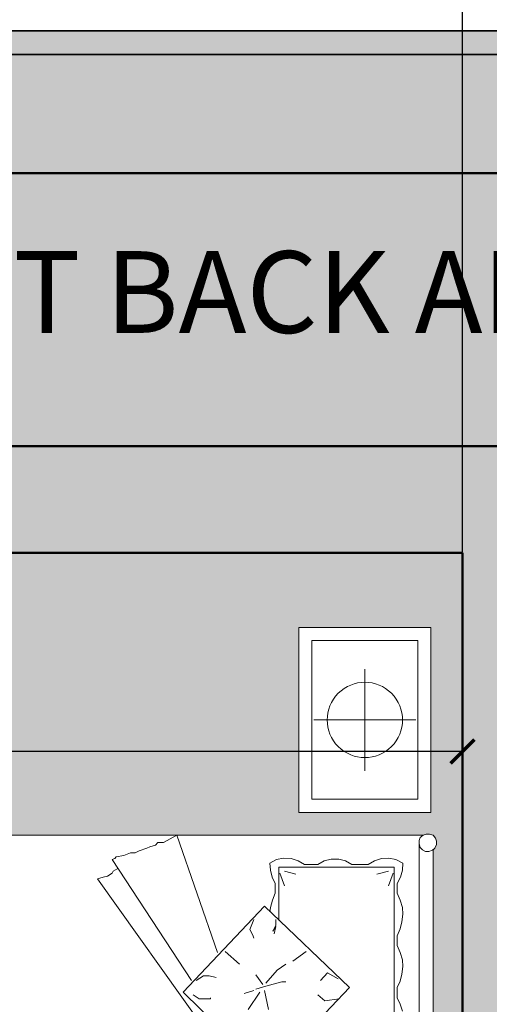
# Model space of a CAD drawing. Units: inches. Extents: x 528 to 2620, y -1066 to 798.
# Tile 16 of 41: x 737 to 776, y 672 to 755. Entities that reach past the tile are written whole.
import ezdxf

# ---------------------------------------------------------------- set-up
doc = ezdxf.new("R2010")
doc.units = ezdxf.units.IN
doc.header["$MEASUREMENT"] = 0
for name, color, linetype, lineweight in [('A-ANNO-DIMS', 2, 'Continuous', 18), ('A-AREA-IDEN', 7, 'Continuous', 18), ('A-FURN', 30, 'Continuous', 18), ('A-WALL', 7, 'Continuous', 50), ('A-WALL-PATT', 8, 'Continuous', 13), ('C-PROP', 5, 'Continuous', 35)]:
    doc.layers.add(name, color=color, linetype=linetype, lineweight=lineweight)
doc.styles.get("Standard").update_dxf_attribs({"font": 'arial.ttf'})
doc.dimstyles.get("Standard").update_dxf_attribs({"dimtxt": 6, "dimasz": 2, "dimexe": 0.18, "dimexo": 0.0625, "dimgap": 0.09, "dimtad": 0, "dimtih": 1, "dimtoh": 1, "dimdec": 1, "dimzin": 0, "dimdsep": 46, "dimlunit": 3, "dimtxsty": 'Standard', "dimblk": 'ARCHTICK', "dimcen": 0.09, "dimadec": 0, "dimazin": 0, "dimtfac": 1, "dimtdec": 1, "dimtofl": 0, "dimtmove": 0, "dimatfit": 3, "dimfxl": 1, "dimtolj": 1, "dimtzin": 0, "dimarcsym": 0})

# ---------------------------------------------------------------- blocks, each defined once
blk = doc.blocks.new('d-bed-3')
at = {"color": 0, "linetype": 'ByBlock'}
for p, q in [((0, 0), (0, -0.5)), ((0.7, 0), (0, 0)), ((0.7, -0.5), (0.7, 0)), ((0.7817, -0.0054), (0.7857, 0.0078)), ((0.7817, -0.0054), (0.7857, 0.0078)), ((0.7857, 0.0078), (0.7968, 0.0166)), ((0.7857, 0.0078), (0.7968, 0.0166)), ((0.7968, 0.0166), (0.8078, 0.0211)), ((0.7968, 0.0166), (0.8078, 0.0211)), ((0.8078, 0.0211), (0.8209, 0.0211)), ((0.8078, 0.0211), (0.8209, 0.0211)), ((0.8209, 0.0211), (0.8349, 0.0144)), ((0.8209, 0.0211), (0.8349, 0.0144)), ((0.8349, 0.0144), (0.8409, 0.0078)), ((0.8349, 0.0144), (0.8429, 0.0056)), ((0.8389, 0.0078), (2.7305, 0.0078)), ((0.8409, 0.0078), (2.7305, 0.0078)), ((0.8429, 0.0056), (0.848, -0.0077)), ((0.7817, -0.0187), (0.7817, -0.0054)), ((0.7817, -0.0187), (0.7817, -0.0054)), ((0.7857, -0.0297), (0.7817, -0.0187)), ((0.7857, -0.0297), (0.7817, -0.0187)), ((0.7857, -2.0939), (0.7857, -0.0297)), ((0.7948, -0.0408), (0.7857, -0.0297)), ((0.7857, -0.032), (0.7857, -2.0939)), ((0.8409, -0.032), (0.8319, -0.0408)), ((0.848, -0.0209), (0.8409, -0.032)), ((0.848, -0.0077), (0.848, -0.0209)), ((0.05, -0.05), (0.05, -0.45)), ((0.65, -0.05), (0.05, -0.05)), ((0.35, -0.0576), (0.35, -0.4424)), ((0.65, -0.45), (0.65, -0.05)), ((0.8058, -0.0452), (0.7948, -0.0408)), ((0.8188, -0.0452), (0.8058, -0.0452)), ((0.8319, -0.0408), (0.8188, -0.0452)), ((2.7525, -0.0452), (0.8188, -0.0452)), ((0.8781, -0.1325), (0.8911, -0.1059)), ((0.8911, -0.1059), (0.9182, -0.1082)), ((0.9182, -0.1082), (0.9443, -0.1148)), ((1.0317, -0.117), (1.0588, -0.1082)), ((1.0588, -0.1082), (1.0849, -0.1059)), ((1.0849, -0.1059), (1.113, -0.1104)), ((1.113, -0.1104), (1.1401, -0.117)), ((1.2295, -0.117), (1.2566, -0.1082)), ((1.2566, -0.1082), (1.2827, -0.1059)), ((1.2827, -0.1059), (1.3108, -0.1104)), ((1.3108, -0.1104), (1.3379, -0.117)), ((1.4253, -0.117), (1.4514, -0.1082)), ((0.8721, -0.159), (0.8781, -0.1325)), ((0.9072, -0.5753), (0.9072, -0.1391)), ((0.9072, -0.1391), (1.6763, -0.1391)), ((0.9293, -0.1435), (0.9775, -0.1612)), ((0.9443, -0.1148), (0.9684, -0.128)), ((0.9684, -0.128), (1.0056, -0.128)), ((1.0056, -0.128), (1.0317, -0.117)), ((1.1401, -0.117), (1.1662, -0.128)), ((1.1662, -0.128), (1.2034, -0.128)), ((1.2034, -0.128), (1.2295, -0.117)), ((1.3379, -0.117), (1.362, -0.128)), ((1.362, -0.128), (1.4012, -0.128)), ((1.4012, -0.128), (1.4253, -0.117)), ((0.8741, -0.1866), (0.8721, -0.159)), ((0.9223, -0.1612), (0.9333, -0.2042)), ((0.8831, -0.2131), (0.8741, -0.1866)), ((0.8962, -0.2374), (0.8831, -0.2131)), ((0.1576, -0.25), (0.5424, -0.25)), ((0.8962, -0.2992), (0.8962, -0.2374)), ((0.8761, -0.3489), (0.8831, -0.3235)), ((0.8831, -0.3235), (0.8962, -0.2992)), ((1.0538, -0.6294), (1.362, -0.3081)), ((1.362, -0.3081), (1.619, -0.5532)), ((0.8761, -0.3776), (0.8761, -0.3489)), ((1.3289, -0.3511), (1.3068, -0.3909)), ((1.4052, -0.3467), (1.4122, -0.4019)), ((0.8831, -0.4041), (0.8761, -0.3776)), ((0.8962, -0.4284), (0.8831, -0.4041)), ((1.3068, -0.3909), (1.3349, -0.4174)), ((1.4122, -0.4019), (1.3901, -0.4284)), ((0.8962, -0.4781), (0.8962, -0.4284)), ((0.05, -0.45), (0.65, -0.45)), ((0.8831, -0.5024), (0.8962, -0.4781)), ((1.2255, -0.4715), (1.2626, -0.5223)), ((0, -0.5), (0.7, -0.5)), ((0.8741, -0.5289), (0.8831, -0.5024)), ((0.9223, -0.5532), (0.9333, -0.5113)), ((0.8721, -0.5576), (0.8741, -0.5289)), ((0.8781, -0.5841), (0.8721, -0.5576)), ((0.9293, -0.5709), (0.9775, -0.5532)), ((1.2957, -0.5819), (1.2737, -0.5488)), ((1.3399, -0.5643), (1.3399, -0.5488)), ((0.8911, -0.6096), (0.8781, -0.5841)), ((1.109, -0.5753), (0.9072, -0.5753)), ((0.9684, -0.5886), (0.9443, -0.6007)), ((1.0056, -0.5886), (0.9684, -0.5886)), ((1.0317, -0.5996), (1.0056, -0.5886)), ((1.105, -0.5864), (1.1271, -0.5864)), ((1.1271, -0.5864), (1.1482, -0.5974)), ((1.1482, -0.5974), (1.1311, -0.5864)), ((1.1311, -0.5864), (1.1592, -0.593)), ((1.3459, -0.625), (1.2957, -0.5819)), ((1.357, -0.625), (1.3399, -0.5643)), ((0.9182, -0.6073), (0.8911, -0.6096)), ((0.9443, -0.6007), (0.9182, -0.6073)), ((1.0588, -0.6073), (1.0317, -0.5996)), ((1.3791, -0.9365), (1.0538, -0.6294)), ((1.0759, -0.6096), (1.0588, -0.6073)), ((1.368, -0.6626), (1.357, -0.625)), ((1.3731, -0.6294), (1.4453, -0.614)), ((1.105, -0.6692), (1.1421, -0.6846)), ((1.1642, -0.6736), (1.1753, -0.6692)), ((1.3138, -0.6626), (1.351, -0.6361)), ((1.3731, -0.6692), (1.3841, -0.7067)), ((1.3791, -0.6471), (1.4453, -0.6913)), ((1.1421, -0.6846), (1.1642, -0.6736)), ((1.2255, -0.7785), (1.2737, -0.7244)), ((1.3791, -0.9365), (1.5357, -0.7763)), ((0.7857, -0.9607), (1.2295, -0.8072)), ((0.9504, -1.2611), (1.5708, -0.8183)), ((1.3178, -0.8382), (1.3239, -0.8117)), ((1.3178, -0.8602), (1.3178, -0.8382)), ((1.4052, -0.8337), (1.4012, -0.8337)), ((1.4052, -0.8768), (1.4052, -0.8337)), ((1.3349, -0.8879), (1.3178, -0.8602)), ((1.3901, -0.8989), (1.4052, -0.8768)), ((0.8781, -1.2059), (1.3349, -0.9055)), ((0.8128, -1.0115), (0.7857, -0.9607)), ((0.8128, -1.0325), (0.8128, -1.0115)), ((0.8239, -1.0414), (0.8128, -1.0325)), ((0.8299, -1.0635), (0.8239, -1.0414)), ((0.8349, -1.0745), (0.8299, -1.0635)), ((0.845, -1.1032), (0.8349, -1.0745)), ((0.852, -1.1187), (0.845, -1.1032)), ((0.852, -1.1363), (0.852, -1.1187)), ((0.863, -1.1617), (0.852, -1.1363)), ((0.867, -1.1905), (0.863, -1.1617)), ((0.8741, -1.1949), (0.867, -1.1905)), ((0.9223, -1.2015), (0.9112, -1.1838)), ((0.8781, -1.2059), (0.8741, -1.1949)), ((0.9293, -1.2059), (0.9223, -1.2015)), ((0.9403, -1.2236), (0.9293, -1.2059)), ((0.9443, -1.2391), (0.9403, -1.2236)), ((0.9504, -1.2611), (0.9443, -1.2391))]:
    blk.add_line(p, q, dxfattribs=at)
blk.add_ellipse((0.35, -0.25), major_axis=(-0.1007, 0.1007), ratio=1, dxfattribs=at)
blk = doc.blocks.new('_ArchTick')
at = {"color": 0, "linetype": 'ByBlock', "const_width": 0.15}
blk.add_lwpolyline([(-0.5, -0.5), (0.5, 0.5)], dxfattribs=at)
blk = doc.blocks.new('*D11')
at = {"layer": 'A-ANNO-DIMS', "color": 0, "lineweight": -2, "transparency": 16777216}
for p, q in [((584.059, 753.985), (584.059, 794.007)), ((584.059, 793.827), (758.88, 793.827)), ((944.059, 793.827), (769.239, 793.827)), ((944.059, 753.985), (944.059, 794.007))]:
    blk.add_line(p, q, dxfattribs=at)
at = {"layer": 'Defpoints', "color": 0, "transparency": 16777216}
for p in [(944.059, 793.827), (584.059, 753.922), (944.059, 753.922)]:
    blk.add_point(p, dxfattribs=at)
at = {"layer": 'A-ANNO-DIMS', "color": 0, "lineweight": -2, "transparency": 16777216, "xscale": 2, "yscale": 2, "zscale": 2, "rotation": 180}
blk.add_blockref('_ArchTick', (584.059, 793.827), dxfattribs=at)
at = {"layer": 'A-ANNO-DIMS', "color": 0, "lineweight": -2, "transparency": 16777216, "xscale": 2, "yscale": 2, "zscale": 2}
blk.add_blockref('_ArchTick', (944.059, 793.827), dxfattribs=at)
at = {"layer": 'A-ANNO-DIMS', "color": 0, "transparency": 16777216, "insert": (764.059, 793.827), "char_height": 6, "attachment_point": 5}
blk.add_mtext("\\A1;30'", dxfattribs=at)
blk = doc.blocks.new('*D25')
at = {"layer": 'A-ANNO-DIMS', "color": 0, "lineweight": -2, "transparency": 16777216}
for p, q in [((629.059, 693.763), (629.059, 693.001)), ((629.059, 693.181), (687.951, 693.181)), ((774.059, 693.181), (715.168, 693.181)), ((774.059, 693.763), (774.059, 693.001))]:
    blk.add_line(p, q, dxfattribs=at)
at = {"layer": 'Defpoints', "color": 0, "transparency": 16777216}
for p in [(629.059, 693.826), (774.059, 693.826), (774.059, 693.181)]:
    blk.add_point(p, dxfattribs=at)
at = {"layer": 'A-ANNO-DIMS', "color": 0, "lineweight": -2, "transparency": 16777216, "xscale": 2, "yscale": 2, "zscale": 2, "rotation": 180}
blk.add_blockref('_ArchTick', (629.059, 693.181), dxfattribs=at)
at = {"layer": 'A-ANNO-DIMS', "color": 0, "lineweight": -2, "transparency": 16777216, "xscale": 2, "yscale": 2, "zscale": 2}
blk.add_blockref('_ArchTick', (774.059, 693.181), dxfattribs=at)
at = {"layer": 'A-ANNO-DIMS', "color": 0, "transparency": 16777216, "insert": (701.559, 693.181), "char_height": 6, "attachment_point": 5}
blk.add_mtext('\\A1;12\'-1.0"', dxfattribs=at)
blk = doc.blocks.new('*D56')
at = {"layer": 'A-ANNO-DIMS', "color": 0, "lineweight": -2, "transparency": 16777216}
for p, q in [((774.059, 709.985), (774.059, 788.102)), ((774.059, 787.922), (778.559, 787.922)), ((778.559, 709.985), (778.559, 788.102)), ((778.559, 787.922), (780.559, 787.922))]:
    blk.add_line(p, q, dxfattribs=at)
at = {"layer": 'Defpoints', "color": 0, "transparency": 16777216}
for p in [(778.559, 787.922), (774.059, 709.922), (778.559, 709.922)]:
    blk.add_point(p, dxfattribs=at)
at = {"layer": 'A-ANNO-DIMS', "color": 0, "lineweight": -2, "transparency": 16777216, "xscale": 2, "yscale": 2, "zscale": 2, "rotation": 180}
blk.add_blockref('_ArchTick', (774.059, 787.922), dxfattribs=at)
at = {"layer": 'A-ANNO-DIMS', "color": 0, "lineweight": -2, "transparency": 16777216, "xscale": 2, "yscale": 2, "zscale": 2}
blk.add_blockref('_ArchTick', (778.559, 787.922), dxfattribs=at)
at = {"layer": 'A-ANNO-DIMS', "color": 0, "transparency": 16777216, "insert": (795.615, 787.922), "char_height": 6, "attachment_point": 5}
blk.add_mtext('\\A1;0\'-4 1/2"', dxfattribs=at)

msp = doc.modelspace()

# ---------------------------------------------------------------- hatches: boundary and pattern name
at = {"layer": 'A-WALL-PATT', "transparency": 33554687}
h = msp.add_hatch(color=256, dxfattribs=at)
h.dxf.hatch_style = 1
h.paths.add_polyline_path([(944.059, 753.922), (584.059, 753.922), (584.059, 208.922), (608.059, 208.922), (608.059, 210.922), (586.059, 210.922), (586.059, 751.922), (942.059, 751.922), (942.059, 210.922), (728.059, 210.922), (728.059, 208.922), (944.059, 208.922)])
h = msp.add_hatch(color=256, dxfattribs=at)
h.dxf.hatch_style = 1
h.paths.add_polyline_path([(942.059, 751.922), (586.059, 751.922), (586.059, 210.922), (608.059, 210.922), (608.059, 220.922), (596.059, 220.922), (596.059, 741.922), (932.059, 741.922), (932.059, 220.922), (770.059, 220.922), (728.059, 220.922), (728.059, 210.922), (942.059, 210.922)])
at = {"layer": 'A-WALL-PATT', "transparency": 33554475}
h = msp.add_hatch(color=256, dxfattribs=at)
h.dxf.hatch_style = 1
h.paths.add_polyline_path([(620.059, 718.922), (908.059, 718.922), (908.059, 268.922), (770.059, 268.922), (770.059, 220.922), (932.059, 220.922), (932.059, 741.922), (596.059, 741.922), (596.059, 391.422), (620.059, 391.422)])
at = {"layer": 'A-WALL-PATT', "transparency": 33554687}
h = msp.add_hatch(color=256, dxfattribs=at)
h.dxf.hatch_style = 1
h.paths.add_polyline_path([(861.059, 273.922), (817.059, 273.922), (817.059, 272.922), (861.059, 272.922)])
h.paths.add_polyline_path([(817.059, 277.922), (815.059, 277.922), (815.059, 268.922), (817.059, 268.922)])
h.paths.add_polyline_path([(908.059, 397.922), (899.059, 397.922), (899.059, 395.922), (908.059, 395.922)])
h.paths.add_polyline_path([(908.059, 443.922), (899.059, 443.922), (899.059, 441.922), (908.059, 441.922)])
h.paths.add_polyline_path([(904.059, 441.922), (903.059, 441.922), (903.059, 397.922), (904.059, 397.922)])
h.paths.add_polyline_path([(625.059, 561.422), (624.059, 561.422), (624.059, 537.422), (625.059, 537.422)])
h.paths.add_polyline_path([(648.747, 334.444), (720.045, 334.444), (720.045, 344.998), (648.747, 344.998)], flags=9)
h.paths.add_polyline_path([(819.733, 323.153), (880.328, 323.153), (880.328, 333.708), (819.733, 333.708)], flags=9)
h.paths.add_polyline_path([(779.898, 680.607), (821.764, 680.607), (821.764, 691.169), (779.898, 691.169)], flags=9)
h.paths.add_polyline_path([(779.876, 692.362), (817.138, 692.362), (817.138, 703.058), (779.876, 703.058)], flags=9)
h.paths.add_polyline_path([(799.994, 453.884), (860.589, 453.884), (860.589, 464.439), (799.994, 464.439)], flags=9)
h.paths.add_polyline_path([(650.866, 539.397), (708.781, 539.397), (708.781, 549.952), (650.866, 549.952)], flags=9)
h.paths.add_polyline_path([(788.504, 612.01), (849.099, 612.01), (849.099, 622.565), (788.504, 622.565)], flags=9)
h.paths.add_polyline_path([(639.539, 648.31), (700.134, 648.31), (700.134, 658.865), (639.539, 658.865)], flags=9)
h.paths.add_polyline_path([(648.913, 346.09), (747.706, 346.09), (747.706, 356.778), (648.913, 356.778)], flags=9)
h.paths.add_polyline_path([(676.857, 450.66), (746.735, 450.66), (746.735, 461.355), (676.857, 461.355)], flags=9)
h.paths.add_polyline_path([(819.711, 334.947), (865.526, 334.947), (865.526, 345.636), (819.711, 345.636)], flags=9)
h.paths.add_polyline_path([(806.298, 467.745), (874.047, 467.745), (874.047, 478.441), (806.298, 478.441)], flags=9)
h.paths.add_polyline_path([(653.235, 552.284), (690.497, 552.284), (690.497, 562.979), (653.235, 562.979)], flags=9)
h.paths.add_polyline_path([(789.903, 623.407), (843.208, 623.407), (843.208, 634.103), (789.903, 634.103)], flags=9)
h.paths.add_polyline_path([(639.773, 662.103), (693.077, 662.103), (693.077, 672.798), (639.773, 672.798)], flags=9)
h.paths.add_polyline_path([(801.587, 242.914), (846.334, 242.914), (846.334, 253.603), (801.587, 253.603)], flags=9)
h.paths.add_polyline_path([(925.362, 593.982), (925.362, 674.057), (914.673, 674.057), (914.673, 593.982)], flags=9)
h.paths.add_polyline_path([(612.559, 593.982), (612.559, 674.057), (601.871, 674.057), (601.871, 593.982)], flags=9)
h.paths.add_polyline_path([(723.31, 726.564), (803.385, 726.564), (803.385, 737.252), (723.31, 737.252)], flags=9)
at = {"layer": 'A-WALL-PATT', "transparency": 33554521}
h = msp.add_hatch(color=256, dxfattribs=at)
h.dxf.hatch_style = 1
h.paths.add_polyline_path([(629.059, 709.922), (677.559, 709.922), (677.559, 718.922), (620.059, 718.922), (620.059, 667.922), (629.059, 667.922)])
h.paths.add_polyline_path([(790.559, 718.922), (725.559, 718.922), (725.559, 709.922), (774.059, 709.922), (774.059, 577.922), (768.481, 577.922), (768.559, 573.422), (774.059, 573.422), (774.059, 567.422), (778.559, 567.422), (778.559, 669.422), (831.059, 669.422), (831.059, 675.922), (826.559, 675.922), (826.559, 673.922), (778.559, 673.922), (778.559, 709.922), (790.559, 709.922)])
h.paths.add_polyline_path([(908.059, 718.922), (879.059, 718.922), (879.059, 709.922), (899.059, 709.922), (899.059, 641.672), (908.059, 641.672)])
h.paths.add_polyline_path([(629.059, 619.922), (620.059, 619.922), (620.059, 561.422), (629.059, 561.422), (629.059, 573.422), (724.059, 573.422), (724.059, 569.422), (728.559, 569.422), (728.559, 577.922), (629.059, 577.922)])
h.paths.add_polyline_path([(779.059, 391.422), (779.059, 400.422), (770.059, 400.422), (764.059, 400.422), (764.059, 397.422), (764.059, 391.422), (770.059, 391.422), (770.059, 268.922), (815.059, 268.922), (815.059, 277.922), (779.059, 277.922), (779.059, 359.767)])
h.paths.add_polyline_path([(908.059, 395.922), (899.059, 395.922), (851.059, 395.922), (851.059, 391.422), (899.059, 391.422), (899.059, 277.922), (863.059, 277.922), (863.059, 268.922), (908.059, 268.922)])
h.paths.add_polyline_path([(908.059, 593.672), (899.059, 593.672), (899.059, 525.422), (778.559, 525.422), (778.559, 527.172), (774.059, 527.172), (774.059, 520.922), (899.059, 520.922), (899.059, 443.922), (908.059, 443.922)])
h.paths.add_polyline_path([(629.059, 520.922), (728.559, 520.922), (728.559, 545.422), (724.059, 545.422), (724.059, 525.422), (629.059, 525.422), (629.059, 537.422), (620.059, 537.422), (620.059, 484.672), (629.059, 484.672)])
h.paths.add_polyline_path([(629.059, 436.672), (620.059, 436.672), (620.059, 391.422), (648.559, 391.422), (648.559, 400.422), (629.059, 400.422)])
h.paths.add_polyline_path([(716.059, 397.422), (716.059, 400.422), (696.559, 400.422), (696.559, 391.422), (716.059, 391.422)])
at = {"layer": 'A-WALL-PATT', "transparency": 33554590}
h = msp.add_hatch(color=256, dxfattribs=at)
h.dxf.hatch_style = 1
h.paths.add_polyline_path([(774.059, 709.922), (629.059, 709.922), (629.059, 577.922), (728.559, 577.922), (728.559, 579.422), (728.559, 619.422), (730.309, 619.422), (730.309, 619.384, -0.401453), (768.559, 579.422), (768.559, 577.922), (774.059, 577.922)])
h.paths.add_polyline_path([(723.896, 686.058), (723.968, 686.064), (723.828, 686.128)], flags=0)
h.paths.add_polyline_path([(722.785, 642.699), (722.893, 642.756), (722.893, 684.992), (722.647, 685.244), (722.647, 685.82), (723.079, 686.262), (723.533, 686.262), (723.968, 686.064), (724.739, 686.128), (770.696, 686.128), (770.78, 686.14), (771.126, 686.266), (771.694, 686.094), (771.94, 685.478), (771.67, 684.904), (771.582, 684.871), (771.582, 642.782), (771.878, 642.514), (771.878, 641.921), (771.511, 641.462), (770.855, 641.462), (770.401, 641.833), (770.401, 641.551), (724.739, 641.551), (723.991, 641.705), (723.443, 641.414), (722.879, 641.585), (722.597, 642.142)], flags=16)
h.paths.add_polyline_path([(723.994, 641.704), (723.994, 641.707), (723.991, 641.705)], flags=0)
h.paths.add_polyline_path([(722.893, 642.732), (722.893, 684.992), (722.647, 685.244), (722.647, 685.82), (723.079, 686.262), (723.287, 686.262), (722.991, 686.172), (722.794, 685.971), (722.647, 685.68), (722.647, 685.434), (722.745, 685.143), (722.942, 684.942), (723.238, 684.807), (723.484, 684.807), (723.779, 684.897), (723.976, 685.098), (724.174, 685.488), (724.124, 685.635), (724.124, 685.249), (723.631, 684.746), (723.631, 642.961), (724.124, 642.514), (724.124, 641.887), (723.656, 641.462), (723.079, 641.462), (722.647, 641.904), (722.647, 642.48)], flags=0)
h.paths.add_polyline_path([(722.647, 642.29), (722.647, 642.044), (722.794, 641.753), (723.079, 641.462), (723.287, 641.462), (722.879, 641.585), (722.597, 642.142)], flags=0)
h.paths.add_polyline_path([(770.745, 686.128), (770.58, 686.128), (770.551, 686.057)], flags=0)
h.paths.add_polyline_path([(743.299, 645.288), (753.227, 659.398), (748.69, 663.75), (753.234, 668.538), (743.299, 682.458), (743.791, 682.592), (744.136, 682.681), (744.53, 682.928), (744.628, 683.084), (745.017, 683.327), (744.53, 684.069), (744.776, 684.158), (744.874, 684.315), (745.514, 684.404), (746.081, 684.651), (746.474, 684.651), (746.819, 684.807), (747.459, 685.031), (747.705, 685.143), (748.198, 685.277), (748.394, 685.523), (748.862, 685.523), (749.994, 686.128), (753.488, 676.03), (757.379, 680.153), (757.791, 679.758), (758.044, 680.645), (758.29, 681.227), (758.29, 682.055), (758.019, 682.592), (757.871, 683.174), (757.822, 683.778), (758.388, 684.069), (758.979, 684.203), (759.619, 684.158), (760.21, 683.957), (760.751, 683.666), (761.859, 683.666), (762.401, 683.957), (762.991, 684.114), (763.631, 684.114), (764.198, 683.957), (764.739, 683.666), (766.118, 683.666), (766.659, 683.957), (767.25, 684.158), (767.865, 684.203), (768.456, 684.069), (769.047, 683.778), (768.998, 683.174), (768.85, 682.592), (768.554, 682.055), (768.554, 681.227), (768.801, 680.645), (769.092, 679.75), (768.948, 678.832), (768.801, 678.228), (768.554, 677.646), (768.554, 676.818), (768.801, 676.237), (769.092, 675.341), (768.948, 674.424), (768.801, 673.82), (768.554, 673.283), (768.554, 672.41), (768.801, 671.873), (768.998, 671.291), (769.047, 670.642), (768.948, 670.016), (768.801, 669.411), (768.554, 668.874), (768.554, 668.002), (768.974, 667.239), (769.047, 666.279), (769.047, 665.563), (768.456, 665.316), (767.865, 665.16), (767.25, 665.16), (766.659, 665.361), (766.118, 665.697), (764.739, 665.697), (763.945, 665.204), (762.991, 665.204), (762.401, 665.361), (761.859, 665.697), (761.005, 665.697), (762.696, 664.086), (760.741, 662.027), (761.859, 662.027), (762.401, 662.318), (763.342, 662.548), (764.247, 662.318), (764.788, 662.027), (766.118, 662.027), (766.659, 662.318), (767.25, 662.519), (767.865, 662.564), (768.505, 662.43), (769.047, 662.116), (769.047, 661.4), (769.047, 660.796), (768.85, 660.214), (768.554, 659.677), (768.554, 658.849), (768.85, 658.267), (768.998, 657.663), (769.069, 656.749), (768.85, 655.851), (768.554, 655.269), (768.554, 654.441), (768.85, 653.859), (769.069, 652.961), (768.998, 652.046), (768.85, 651.442), (768.554, 650.905), (768.554, 650.032), (768.85, 649.495), (768.998, 648.914), (769.047, 648.265), (768.998, 647.638), (768.85, 647.034), (768.554, 646.497), (768.554, 645.624), (768.85, 645.087), (769.047, 644.55), (769.047, 643.901), (768.505, 643.655), (767.865, 643.521), (767.25, 643.521), (766.659, 643.722), (766.118, 644.058), (764.788, 644.058), (764.247, 643.722), (763.342, 643.492), (762.401, 643.722), (761.859, 644.058), (760.801, 644.058), (760.259, 643.722), (759.668, 643.521), (759.028, 643.521), (758.388, 643.655), (757.871, 643.901), (757.871, 644.55), (758.044, 645.087), (758.339, 645.624), (758.339, 646.497), (758.044, 647.034), (757.921, 647.638), (757.866, 648.059), (757.379, 647.593), (753.422, 651.773), (749.994, 641.618), (749.502, 641.708), (749.354, 641.954), (748.542, 642.446), (747.311, 642.939), (746.652, 642.939), (746.327, 643.185), (745.514, 643.565), (744.53, 643.655), (745.011, 644.4), (744.628, 644.639), (744.136, 644.886), (743.791, 645.132)], flags=0)
h.paths.add_polyline_path([(755.656, 654.933), (756.542, 654.687), (757.527, 654.329), (756.641, 654.575)], flags=0)
h.paths.add_polyline_path([(758.339, 649.204), (758.339, 648.712), (758.585, 644.304), (758.585, 648.802)], flags=0)
h.paths.add_polyline_path([(758.339, 649.294), (758.093, 649.697), (758.359, 649.165)], flags=0)
h.paths.add_polyline_path([(755.656, 672.79), (756.493, 673.037), (757.358, 673.351), (757.353, 673.358), (756.641, 673.149)], flags=0)
h.paths.add_polyline_path([(760.264, 639.641), (771.408, 639.641), (771.408, 624.039), (760.264, 624.039)], flags=16)
h.paths.add_polyline_path([(761.378, 638.526), (770.294, 638.526), (770.294, 625.153), (761.378, 625.153)], flags=0)
edge = h.paths.add_edge_path(flags=0)
edge.add_ellipse((765.836, 631.84), major_axis=(-2.245, 2.245), ratio=1, start_angle=-45, end_angle=45, ccw=False)
edge.add_ellipse((765.836, 631.84), major_axis=(-2.245, 2.245), ratio=1, start_angle=-135, end_angle=-45, ccw=False)
edge.add_ellipse((765.836, 631.84), major_axis=(-2.245, 2.245), ratio=1, start_angle=135, end_angle=-135, ccw=False)
edge.add_ellipse((765.836, 631.84), major_axis=(-2.245, 2.245), ratio=1, start_angle=45, end_angle=135, ccw=False)
h.paths.add_polyline_path([(758.585, 683.42), (758.585, 678.922), (758.373, 678.575), (758.339, 678.43), (758.093, 678.049), (758.339, 678.519), (758.339, 679.011)], flags=0)
h.paths.add_polyline_path([(760.264, 688.038), (760.264, 703.64), (771.408, 703.64), (771.408, 688.038)], flags=16)
h.paths.add_polyline_path([(770.401, 685.389), (770.401, 685.846), (770.855, 686.217), (771.511, 686.217), (771.878, 685.758), (771.878, 685.165), (771.582, 684.897), (771.582, 642.782), (771.878, 642.514), (771.878, 641.921), (771.511, 641.462), (770.855, 641.462), (770.401, 641.833), (770.401, 642.29)], flags=0)
h.paths.add_polyline_path([(770.532, 642.678), (771.052, 643.009), (771.67, 642.775), (771.94, 642.201), (771.694, 641.585), (771.126, 641.413), (770.551, 641.622), (770.347, 642.132)], flags=16)
h.paths.add_polyline_path([(761.378, 689.152), (761.378, 702.526), (770.294, 702.526), (770.294, 689.152)], flags=0)
edge = h.paths.add_edge_path(flags=0)
edge.add_ellipse((765.836, 695.839), major_axis=(2.245, 2.245), ratio=1, start_angle=405, end_angle=495, ccw=False)
edge.add_ellipse((765.836, 695.839), major_axis=(2.245, 2.245), ratio=1, start_angle=675, end_angle=765, ccw=False)
edge.add_ellipse((765.836, 695.839), major_axis=(2.245, 2.245), ratio=1, start_angle=585, end_angle=675, ccw=False)
edge.add_ellipse((765.836, 695.839), major_axis=(2.245, 2.245), ratio=1, start_angle=495, end_angle=585, ccw=False)
h.paths.add_polyline_path([(770.696, 684.897), (770.942, 684.74), (771.41, 684.74), (771.73, 685.031), (771.878, 685.344), (771.878, 685.635), (771.694, 686.094), (771.582, 686.128), (771.878, 685.758), (771.878, 685.165), (771.41, 684.74), (770.849, 684.74)], flags=0)
h.paths.add_polyline_path([(899.059, 709.922), (831.059, 709.922), (831.059, 699.922), (829.809, 699.922), (829.809, 675.922), (831.059, 675.922), (831.059, 669.422), (778.559, 669.422), (778.559, 567.172), (780.059, 567.172), (820.059, 567.172), (820.059, 565.422), (820.021, 565.422, -0.401453), (780.059, 527.172), (778.559, 527.172), (778.559, 525.422), (899.059, 525.422)])
h.paths.add_polyline_path([(849.197, 636.014), (849.269, 636.02), (849.129, 636.084)], flags=0)
h.paths.add_polyline_path([(848.193, 634.948), (847.947, 635.2), (847.947, 635.776), (848.379, 636.218), (848.833, 636.218), (849.269, 636.02), (850.039, 636.084), (895.996, 636.084), (896.081, 636.096), (896.426, 636.222), (896.995, 636.05), (897.241, 635.434), (896.97, 634.86), (896.883, 634.827), (896.883, 592.738), (897.178, 592.47), (897.178, 591.877), (896.811, 591.418), (896.155, 591.418), (895.701, 591.789), (895.701, 591.507), (850.039, 591.507), (849.292, 591.661), (848.744, 591.37), (848.18, 591.541), (847.897, 592.098), (848.086, 592.655), (848.193, 592.712)], flags=16)
h.paths.add_polyline_path([(849.294, 591.66), (849.295, 591.663), (849.292, 591.661)], flags=16)
h.paths.add_polyline_path([(848.193, 634.948), (847.947, 635.2), (847.947, 635.776), (848.379, 636.218), (848.587, 636.218), (848.292, 636.128), (848.095, 635.927), (847.947, 635.636), (847.947, 635.39), (848.046, 635.099), (848.243, 634.897), (848.538, 634.763), (848.784, 634.763), (849.079, 634.853), (849.276, 635.054), (849.474, 635.444), (849.424, 635.591), (849.424, 635.205), (848.932, 634.702), (848.932, 592.917), (849.424, 592.47), (849.424, 591.843), (848.956, 591.418), (848.379, 591.418), (847.947, 591.86), (847.947, 592.436), (848.193, 592.688)], flags=0)
h.paths.add_polyline_path([(847.947, 592.246), (847.947, 592), (848.095, 591.709), (848.379, 591.418), (848.587, 591.418), (848.18, 591.541), (847.897, 592.098)], flags=16)
h.paths.add_polyline_path([(896.046, 636.084), (895.88, 636.084), (895.852, 636.013)], flags=0)
h.paths.add_polyline_path([(868.599, 632.414), (869.092, 632.548), (869.436, 632.637), (869.83, 632.884), (869.929, 633.04), (870.318, 633.283), (869.83, 634.025), (870.076, 634.114), (870.175, 634.271), (870.815, 634.36), (871.381, 634.607), (871.775, 634.607), (872.119, 634.763), (872.759, 634.987), (873.006, 635.099), (873.498, 635.233), (873.695, 635.479), (874.163, 635.479), (875.295, 636.084), (878.788, 625.986), (882.679, 630.109), (883.091, 629.714), (883.344, 630.601), (883.59, 631.183), (883.59, 632.011), (883.319, 632.548), (883.172, 633.13), (883.123, 633.734), (883.689, 634.025), (884.279, 634.159), (884.919, 634.114), (885.51, 633.913), (886.052, 633.622), (887.159, 633.622), (887.701, 633.913), (888.292, 634.07), (888.932, 634.07), (889.498, 633.913), (890.039, 633.622), (891.418, 633.622), (891.959, 633.913), (892.55, 634.114), (893.166, 634.159), (893.756, 634.025), (894.347, 633.734), (894.298, 633.13), (894.15, 632.548), (893.855, 632.011), (893.855, 631.183), (894.101, 630.601), (894.393, 629.706), (894.249, 628.788), (894.101, 628.184), (893.855, 627.602), (893.855, 626.774), (894.101, 626.193), (894.393, 625.297), (894.249, 624.38), (894.101, 623.776), (893.855, 623.239), (893.855, 622.366), (894.101, 621.829), (894.298, 621.247), (894.347, 620.598), (894.249, 619.972), (894.101, 619.367), (893.855, 618.83), (893.855, 617.958), (894.274, 617.195), (894.347, 616.235), (894.347, 615.518), (893.756, 615.272), (893.166, 615.116), (892.55, 615.116), (891.959, 615.317), (891.418, 615.653), (890.039, 615.653), (889.245, 615.16), (888.292, 615.16), (887.701, 615.317), (887.159, 615.653), (886.305, 615.653), (887.996, 614.042), (886.041, 611.983), (887.159, 611.983), (887.701, 612.274), (888.642, 612.504), (889.547, 612.274), (890.089, 611.983), (891.418, 611.983), (891.959, 612.274), (892.55, 612.475), (893.166, 612.52), (893.806, 612.386), (894.347, 612.072), (894.347, 611.356), (894.347, 610.752), (894.15, 610.17), (893.855, 609.633), (893.855, 608.805), (894.15, 608.223), (894.298, 607.619), (894.37, 606.705), (894.15, 605.807), (893.855, 605.225), (893.855, 604.397), (894.15, 603.815), (894.37, 602.917), (894.298, 602.002), (894.15, 601.398), (893.855, 600.861), (893.855, 599.988), (894.15, 599.451), (894.298, 598.87), (894.347, 598.221), (894.298, 597.594), (894.15, 596.99), (893.855, 596.453), (893.855, 595.58), (894.15, 595.043), (894.347, 594.506), (894.347, 593.857), (893.806, 593.611), (893.166, 593.477), (892.55, 593.477), (891.959, 593.678), (891.418, 594.014), (890.089, 594.014), (889.547, 593.678), (888.642, 593.448), (887.701, 593.678), (887.159, 594.014), (886.101, 594.014), (885.559, 593.678), (884.969, 593.477), (884.329, 593.477), (883.689, 593.611), (883.172, 593.857), (883.172, 594.506), (883.344, 595.043), (883.639, 595.58), (883.639, 596.453), (883.344, 596.99), (883.221, 597.594), (883.167, 598.015), (882.679, 597.549), (878.722, 601.729), (875.295, 591.574), (874.803, 591.664), (874.655, 591.91), (873.843, 592.402), (872.612, 592.895), (871.952, 592.895), (871.627, 593.141), (870.815, 593.521), (869.83, 593.611), (870.311, 594.356), (869.929, 594.595), (869.436, 594.842), (869.092, 595.088), (868.599, 595.244), (878.528, 609.354), (873.99, 613.706), (878.535, 618.494)], flags=0)
h.paths.add_polyline_path([(880.956, 622.746), (881.793, 622.993), (882.659, 623.307), (882.654, 623.314), (881.941, 623.104)], flags=0)
h.paths.add_polyline_path([(880.956, 604.889), (881.843, 604.643), (882.827, 604.285), (881.941, 604.531)], flags=16)
h.paths.add_polyline_path([(883.393, 628.005), (883.639, 628.475), (883.639, 628.967), (883.886, 633.376), (883.886, 628.878), (883.674, 628.531), (883.639, 628.386)], flags=0)
h.paths.add_polyline_path([(883.639, 599.16), (883.639, 598.668), (883.886, 594.26), (883.886, 598.758)], flags=16)
h.paths.add_polyline_path([(883.639, 599.25), (883.393, 599.653), (883.659, 599.121)], flags=16)
h.paths.add_polyline_path([(885.564, 637.994), (885.564, 653.596), (896.709, 653.596), (896.709, 637.994)], flags=16)
h.paths.add_polyline_path([(885.564, 589.597), (896.709, 589.597), (896.709, 573.995), (885.564, 573.995)], flags=16)
h.paths.add_polyline_path([(886.679, 639.108), (886.679, 652.482), (895.594, 652.482), (895.594, 639.108)], flags=0)
h.paths.add_polyline_path([(886.679, 588.482), (895.594, 588.482), (895.594, 575.109), (886.679, 575.109)], flags=0)
edge = h.paths.add_edge_path(flags=0)
edge.add_ellipse((891.136, 645.795), major_axis=(2.245, 2.245), ratio=1, start_angle=405, end_angle=495, ccw=False)
edge.add_ellipse((891.136, 645.795), major_axis=(2.245, 2.245), ratio=1, start_angle=675, end_angle=765, ccw=False)
edge.add_ellipse((891.136, 645.795), major_axis=(2.245, 2.245), ratio=1, start_angle=585, end_angle=675, ccw=False)
edge.add_ellipse((891.136, 645.795), major_axis=(2.245, 2.245), ratio=1, start_angle=495, end_angle=585, ccw=False)
edge = h.paths.add_edge_path(flags=0)
edge.add_ellipse((891.136, 581.796), major_axis=(-2.245, 2.245), ratio=1, start_angle=-45, end_angle=45, ccw=False)
edge.add_ellipse((891.136, 581.796), major_axis=(-2.245, 2.245), ratio=1, start_angle=-135, end_angle=-45, ccw=False)
edge.add_ellipse((891.136, 581.796), major_axis=(-2.245, 2.245), ratio=1, start_angle=135, end_angle=-135, ccw=False)
edge.add_ellipse((891.136, 581.796), major_axis=(-2.245, 2.245), ratio=1, start_angle=45, end_angle=135, ccw=False)
h.paths.add_polyline_path([(895.701, 635.345), (895.701, 635.802), (896.155, 636.173), (896.811, 636.173), (897.178, 635.714), (897.178, 635.121), (896.883, 634.853), (896.883, 592.738), (897.178, 592.47), (897.178, 591.877), (896.811, 591.418), (896.155, 591.418), (895.701, 591.789), (895.701, 592.246)], flags=0)
h.paths.add_polyline_path([(895.996, 634.853), (896.243, 634.696), (896.71, 634.696), (897.03, 634.987), (897.178, 635.3), (897.178, 635.591), (896.995, 636.05), (896.883, 636.084), (897.178, 635.714), (897.178, 635.121), (896.71, 634.696), (896.15, 634.696)], flags=0)
h.paths.add_polyline_path([(895.832, 592.634), (896.353, 592.965), (896.97, 592.731), (897.241, 592.157), (896.995, 591.541), (896.426, 591.369), (895.852, 591.578), (895.648, 592.088)], flags=16)
h.paths.add_polyline_path([(725.255, 569.422), (724.059, 569.422), (724.059, 573.422), (629.059, 573.422), (629.059, 525.422), (724.059, 525.422), (724.059, 545.422), (725.255, 545.422)])
h.paths.add_polyline_path([(820.021, 565.422), (780.059, 565.422), (780.059, 567.172), (774.059, 567.172), (774.059, 567.422), (774.059, 573.422), (768.559, 573.422), (768.481, 577.922), (768.559, 577.922), (768.559, 579.422, 0.401453), (730.309, 619.384), (730.309, 579.422), (728.559, 579.422), (728.559, 573.422), (728.559, 569.422), (727.255, 569.422), (727.255, 545.422), (728.559, 545.422), (728.559, 520.922), (665.059, 520.922), (665.059, 436.422), (716.059, 436.422), (716.059, 421.422), (717.809, 421.422), (717.809, 421.358, -0.392996), (740.059, 397.422, -0.392996), (762.309, 421.358), (762.309, 421.422), (764.059, 421.422), (764.059, 400.422), (770.059, 400.422), (779.059, 400.422), (779.059, 391.422), (779.059, 359.767), (795.432, 359.767), (795.432, 294.295), (893.669, 294.295), (893.669, 277.922), (899.059, 277.922), (899.059, 391.422), (851.059, 391.422), (851.059, 395.922), (899.059, 395.922), (899.059, 443.922), (899.059, 520.922), (774.059, 520.922), (774.059, 527.172), (778.559, 527.172), (780.059, 527.172, 0.401453)])
h.paths.add_polyline_path([(774.059, 519.657), (842.122, 519.657), (842.122, 505.072), (788.644, 505.072), (788.644, 474.079), (788.644, 470.433, -0.883215), (779.529, 456.663), (774.971, 456.663, -0.414214), (774.059, 457.575)], flags=16)
h.paths.add_polyline_path([(775.883, 517.834), (840.299, 517.834), (840.299, 514.188), (788.644, 514.188), (788.644, 484.41), (779.529, 484.41), (779.529, 474.079), (775.883, 474.079)], flags=0)
h.paths.add_polyline_path([(706.7, 501.564, -0.254069), (706.7, 493.021), (698.31, 492.555), (698.31, 502.031)], flags=16)
h.paths.add_polyline_path([(691.334, 515.692), (691.8, 507.301), (682.325, 507.301), (682.791, 515.692, -0.254069)], flags=16)
h.paths.add_polyline_path([(695.485, 504.685), (695.485, 479.416), (678.64, 479.416), (678.64, 504.685)], flags=16)
h.paths.add_polyline_path([(706.7, 489.602, -0.254069), (706.7, 481.058), (698.31, 480.592), (698.31, 490.068)], flags=16)
h.paths.add_polyline_path([(675.815, 502.031), (675.815, 492.555), (667.425, 493.021, -0.254069), (667.425, 501.564)], flags=16)
h.paths.add_polyline_path([(691.8, 476.8), (691.334, 468.409, -0.254069), (682.791, 468.409), (682.325, 476.8)], flags=16)
h.paths.add_polyline_path([(675.815, 490.068), (675.815, 480.592), (667.425, 481.058, -0.254069), (667.425, 489.602)], flags=16)
h.paths.add_polyline_path([(764.059, 397.422), (762.309, 397.422), (762.309, 421.358, 0.392996), (740.059, 397.422, 0.392996), (717.809, 421.358), (717.809, 397.422), (716.059, 397.422), (716.059, 391.422), (716.059, 385.422), (764.059, 385.422), (764.059, 391.422)], flags=17)
h.paths.add_polyline_path([(716.059, 436.422), (705.859, 436.422), (705.859, 418.422), (716.059, 418.422), (716.059, 421.422)], flags=17)
h.paths.add_polyline_path([(716.059, 418.422), (705.859, 418.422), (705.859, 400.422), (716.059, 400.422)], flags=17)
h.paths.add_polyline_path([(705.859, 418.422), (695.659, 418.422), (695.659, 400.422), (696.559, 400.422), (705.859, 400.422)], flags=17)
h.paths.add_polyline_path([(705.859, 436.422), (695.659, 436.422), (695.659, 418.422), (705.859, 418.422)], flags=17)
h.paths.add_polyline_path([(695.659, 418.422), (685.459, 418.422), (685.459, 400.422), (695.659, 400.422)], flags=17)
h.paths.add_polyline_path([(695.659, 436.422), (685.459, 436.422), (685.459, 418.422), (695.659, 418.422)], flags=17)
h.paths.add_polyline_path([(685.459, 418.422), (675.259, 418.422), (675.259, 400.422), (685.459, 400.422)], flags=17)
h.paths.add_polyline_path([(685.459, 436.422), (675.259, 436.422), (675.259, 418.422), (685.459, 418.422)], flags=17)
h.paths.add_polyline_path([(675.259, 436.422), (665.059, 436.422), (665.059, 418.422), (675.259, 418.422)])
h.paths.add_polyline_path([(675.259, 418.422), (665.059, 418.422), (665.059, 400.422), (675.259, 400.422)])
h.paths.add_polyline_path([(665.059, 418.422), (646.967, 418.422), (646.991, 436.422), (629.059, 436.422), (629.059, 400.422), (665.059, 400.422)])
h.paths.add_polyline_path([(665.059, 436.422), (646.991, 436.422), (646.967, 418.422), (665.059, 418.422)], flags=17)
h.paths.add_polyline_path([(647.005, 446.622), (629.059, 446.622), (629.059, 436.672), (629.059, 436.422), (646.991, 436.422)])
h.paths.add_polyline_path([(665.059, 446.622), (647.005, 446.622), (646.991, 436.422), (665.059, 436.422)])
h.paths.add_polyline_path([(647.019, 456.822), (629.059, 456.822), (629.059, 446.622), (647.005, 446.622)])
h.paths.add_polyline_path([(665.059, 456.822), (647.019, 456.822), (647.005, 446.622), (665.059, 446.622)])
h.paths.add_polyline_path([(647.032, 467.022), (629.059, 467.022), (629.059, 456.822), (647.019, 456.822)])
h.paths.add_polyline_path([(665.059, 467.022), (647.032, 467.022), (647.019, 456.822), (665.059, 456.822)])
h.paths.add_polyline_path([(665.059, 477.222), (647.046, 477.222), (647.032, 467.022), (665.059, 467.022)])
h.paths.add_polyline_path([(647.046, 477.222), (629.059, 477.222), (629.059, 467.022), (647.032, 467.022)])
h.paths.add_polyline_path([(647.059, 487.222), (629.059, 487.222), (629.059, 477.222), (647.046, 477.222), (647.048, 479.019), (645.53, 483.246), (640.877, 480.371)])
h.paths.add_polyline_path([(665.059, 520.922), (629.059, 520.922), (629.059, 487.222), (647.059, 487.222), (665.059, 487.222)])
h.paths.add_polyline_path([(665.059, 487.222), (647.059, 487.222), (653.224, 480.355), (648.578, 483.242), (647.048, 479.019), (647.046, 477.222), (665.059, 477.222)])

# ---------------------------------------------------------------- linework, layer by layer
at = {"layer": 'A-WALL'}
for p, q in [((932.059, 741.922), (596.059, 741.922)), ((908.059, 718.922), (620.059, 718.922)), ((774.059, 709.922), (629.059, 709.922)), ((774.059, 709.922), (774.059, 577.922))]:
    msp.add_line(p, q, dxfattribs=at)
at = {"layer": 'C-PROP'}
for points in [[(728.059, 208.922), (944.059, 208.922), (944.059, 753.922), (584.059, 753.922), (584.059, 208.922), (608.059, 208.922)], [(728.059, 210.922), (942.059, 210.922), (942.059, 751.922), (586.059, 751.922), (586.059, 210.922), (608.059, 210.922)]]:
    msp.add_lwpolyline(points, dxfattribs=at)
msp.add_lwpolyline([(596.059, 741.922), (596.059, 220.922), (932.059, 220.922), (932.059, 741.922)], close=True, dxfattribs=at)

# ---------------------------------------------------------------- block references
at = {"layer": 'A-FURN', "xscale": 22.28859121186505, "yscale": 22.28859121186505, "zscale": 22.28859121186505, "rotation": 270}
msp.add_blockref('d-bed-3', (771.408, 703.64), dxfattribs=at)

# ---------------------------------------------------------------- texts
at = {"layer": 'A-AREA-IDEN'}
msp.add_text('SET BACK AREA', height=6.89074, dxfattribs=at).set_placement((725.091, 728.463))

# ---------------------------------------------------------------- dimensions: what is measured, and where the dimension line sits
at = {"layer": 'A-ANNO-DIMS'}
for base, p1, p2, override, picture, middle in [((944.059, 793.827), (584.059, 753.922), (944.059, 753.922), {"dimclrd": 0, "dimclre": 0, "dimclrt": 0}, '*D11', (764.059, 793.827)), ((778.559, 787.922), (774.059, 709.922), (778.559, 709.922), {"dimdec": 1, "dimlfac": 1, "dimrnd": 0, "dimzin": 1, "dimdsep": 46, "dimlunit": 4, "dimfrac": 2}, '*D56', (795.615, 787.922)), ((774.059, 693.181), (629.059, 693.826), (774.059, 693.826), {"dimclrd": 0, "dimclre": 0, "dimclrt": 0}, '*D25', (701.559, 693.181))]:
    dim = msp.add_linear_dim(base=base, p1=p1, p2=p2, dimstyle='Standard', override=override, dxfattribs=at)
    dim.commit()
    dim.dimension.update_dxf_attribs({"geometry": picture, "text_midpoint": middle})

doc.saveas('drawing.dxf')
